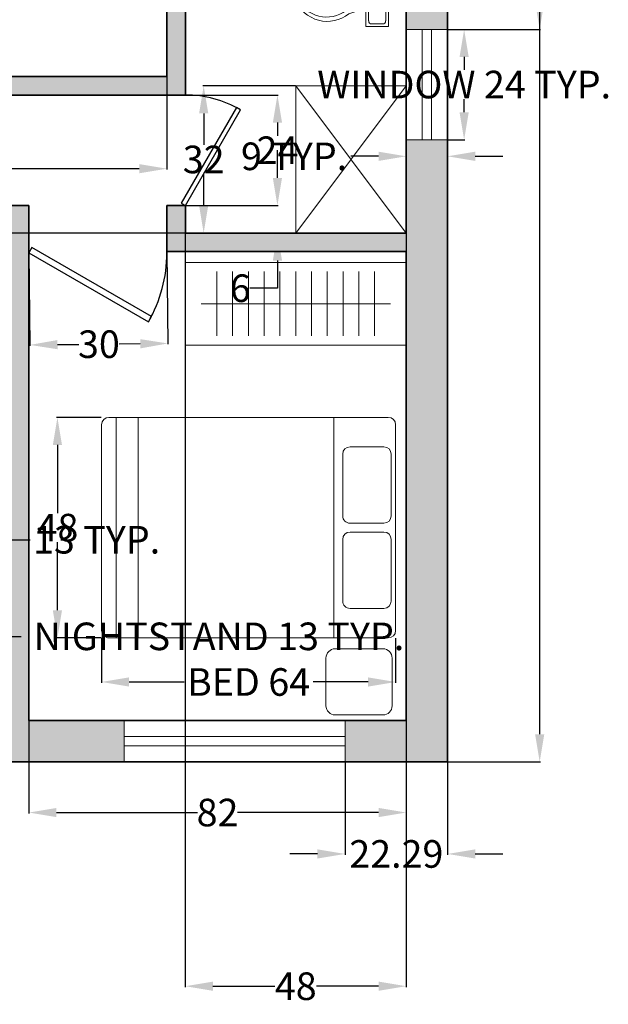
# Model space of a CAD drawing. Units: inches. Extents: x -26 to 363, y -399 to 37.
# Tile 2 of 4: x 232 to 360, y -399 to -185. Entities that reach past the tile are written whole.
import ezdxf

# ---------------------------------------------------------------- set-up
doc = ezdxf.new("R2010")
doc.units = ezdxf.units.IN
doc.header["$MEASUREMENT"] = 0
for name, color, linetype, lineweight in [('A-ANNO-DIMS', 2, 'Continuous', 18), ('A-DOOR', 3, 'Continuous', 25), ('A-FLOR-CASE', 8, 'Continuous', 18), ('A-FLOR-FIXT', 9, 'Continuous', 18), ('A-FURN', 8, 'Continuous', 18), ('A-GLAZ', 4, 'Continuous', 18), ('A-WALL', 7, 'Continuous', 35), ('A-WALL-PATT', 251, 'Continuous', 13)]:
    doc.layers.add(name, color=color, linetype=linetype, lineweight=lineweight)
doc.styles.get("Standard").update_dxf_attribs({"font": 'arial.ttf'})
doc.dimstyles.get("Standard").update_dxf_attribs({"dimtxt": 6, "dimasz": 6, "dimexe": 0.18, "dimexo": 0.0625, "dimgap": 0.09, "dimtad": 0, "dimtih": 1, "dimtoh": 1, "dimdec": 0, "dimzin": 0, "dimdsep": 46, "dimlunit": 4, "dimtxsty": 'Standard', "dimcen": 0.09, "dimadec": 0, "dimazin": 0, "dimtfac": 1, "dimtdec": 0, "dimtofl": 0, "dimtmove": 0, "dimatfit": 3, "dimfxl": 1, "dimtolj": 1, "dimtzin": 0, "dimarcsym": 0})

# ---------------------------------------------------------------- blocks, each defined once
blk = doc.blocks.new('*U3')
for p, q in [((0, 0), (0, 6)), ((40, 0), (40, 6))]:
    blk.add_line(p, q)
blk.add_lwpolyline([(0, 0), (34.64, -20), (35.52, -18.48), (0.87, 1.52)], close=True)
blk.add_arc((0, 0), 40, 330, 0)
blk = doc.blocks.new('Toilet - top')
for p, q in [((9.5, -6), (9.5, -2)), ((-10, -8.5), (-8, -8.5)), ((-10, -9.5), (-10, -8.5)), ((-7, -9.5), (-10, -9.5)), ((-8, -8.5), (-8, -8)), ((-7, -8), (-7, -9.5)), ((-4, -8), (-6, -14)), ((4, -8), (6, -14)), ((4, -14), (-4, -14))]:
    blk.add_line(p, q)
blk.add_lwpolyline([(10.5, -8), (10.5, 0), (-10.5, 0), (-10.5, -8)], close=True)
for points in [[(-9.5, -2), (-9.5, -6)], [(8.5, -1), (-8.5, -1)], [(-8.5, -7), (8.5, -7)]]:
    blk.add_lwpolyline(points)
for centre, radius, start, end in [((-8.62, -1.88), 0.884, 81.8699, 188.1301), ((8.62, -1.88), 0.884, 351.8699, 98.1301), ((-8.62, -6.12), 0.884, 171.8699, 278.1301), ((8.62, -6.12), 0.884, 261.8699, 8.1301), ((3.52, -21.58), 12.17, 141.4691, 247.9714), ((4.2, -21.82), 11.33, 136.3677, 238.9468), ((-3.52, -21.58), 12.17, 292.0284, 38.5307), ((-4.2, -21.82), 11.33, 301.053, 43.6321), ((0, -27.88), 4, 245.7318, 294.2682), ((0, -29), 4, 254.8605, 285.1395)]:
    blk.add_arc(centre, radius, start, end)
blk = doc.blocks.new('Bed - Queen')
for p, q in [((2, 0), (57.99999, 0)), ((0, -78.00003), (0, -2)), ((9.99999, -1.2), (26.79998, -1.2)), ((33.19999, -1.2), (49.99999, -1.2)), ((59.99999, -2), (59.99999, -78.00003)), ((7.99999, -12.4), (7.99999, -3.2)), ((28.79998, -3.2), (28.79998, -12.4)), ((31.19999, -12.4), (31.19999, -3.2)), ((51.99999, -3.2), (51.99999, -12.4)), ((9.99999, -14.4), (26.79998, -14.4)), ((33.19999, -14.4), (49.99999, -14.4)), ((59.99999, -16.8), (0, -16.8)), ((59.99999, -70.00003), (0, -70.00003)), ((59.99999, -76.00003), (0, -76.00003)), ((57.99999, -80.00003), (2, -80.00003))]:
    blk.add_line(p, q)
for centre, start, end in [((2, -2), 90, 180), ((57.99999, -2), 0, 90), ((9.99999, -3.2), 90, 180), ((26.79998, -3.2), 0, 90), ((33.19999, -3.2), 90, 180), ((49.99999, -3.2), 0, 90), ((9.99999, -12.4), 180, 270), ((26.79998, -12.4), 270, 0), ((33.19999, -12.4), 180, 270), ((49.99999, -12.4), 270, 0), ((2, -78.00003), 180, 270), ((57.99999, -78.00003), 270, 0)]:
    blk.add_arc(centre, 2, start, end)
blk = doc.blocks.new('WIN-48IN')
for p, q in [((0, 0), (0, 9)), ((48, 9), (48, 0)), ((48, 5.5), (0, 5.5)), ((48, 3.5), (0, 3.5))]:
    blk.add_line(p, q)
blk = doc.blocks.new('WIN-24IN')
for p, q in [((0, 24), (9, 24)), ((3.5, 24), (3.5, 0)), ((5.5, 24), (5.5, 0)), ((9, 0), (0, 0))]:
    blk.add_line(p, q)
blk = doc.blocks.new('*D23')
at = {"layer": 'A-ANNO-DIMS', "color": 0, "lineweight": -2, "transparency": 16777216}
for p, q in [((250.11, -319.65), (250.11, -329.36)), ((314.03, -319.65), (314.03, -329.36)), ((256.11, -329.18), (268.05, -329.18)), ((308.03, -329.18), (296.09, -329.18))]:
    blk.add_line(p, q, dxfattribs=at)
at = {"layer": 'A-ANNO-DIMS', "color": 0, "transparency": 16777216}
for points in [[(256.11, -328.18), (256.11, -330.18), (250.11, -329.18)], [(308.03, -328.18), (308.03, -330.18), (314.03, -329.18)]]:
    blk.add_solid(points, dxfattribs=at)
at = {"layer": 'Defpoints', "color": 0, "transparency": 16777216}
for p in [(250.11, -319.59), (314.03, -319.59), (314.03, -329.18)]:
    blk.add_point(p, dxfattribs=at)
at = {"layer": 'A-ANNO-DIMS', "color": 0, "transparency": 16777216, "insert": (282.07, -329.18), "char_height": 6, "attachment_point": 5}
blk.add_mtext('\\A1;BED 64', dxfattribs=at)
blk = doc.blocks.new('*D24')
at = {"layer": 'A-ANNO-DIMS', "color": 0, "lineweight": -2, "transparency": 16777216}
for p, q in [((250.04, -271.64), (240.34, -271.64)), ((240.52, -277.64), (240.52, -292.46)), ((240.52, -313.59), (240.52, -298.77)), ((250.04, -319.59), (240.34, -319.59))]:
    blk.add_line(p, q, dxfattribs=at)
at = {"layer": 'A-ANNO-DIMS', "color": 0, "transparency": 16777216}
for points in [[(239.52, -277.64), (241.52, -277.64), (240.52, -271.64)], [(239.52, -313.59), (241.52, -313.59), (240.52, -319.59)]]:
    blk.add_solid(points, dxfattribs=at)
at = {"layer": 'Defpoints', "color": 0, "transparency": 16777216}
for p in [(250.11, -271.64), (240.52, -319.59), (250.11, -319.59)]:
    blk.add_point(p, dxfattribs=at)
at = {"layer": 'A-ANNO-DIMS', "color": 0, "transparency": 16777216, "insert": (240.52, -295.62), "char_height": 6, "attachment_point": 5}
blk.add_mtext('\\A1;48', dxfattribs=at)
blk = doc.blocks.new('*D29')
at = {"layer": 'A-ANNO-DIMS', "color": 0, "lineweight": -2, "transparency": 16777216}
for p, q in [((325.39, -187.28), (329.1, -187.28)), ((328.92, -193.28), (328.92, -196.09)), ((328.92, -205.28), (328.92, -202.48)), ((325.39, -211.28), (329.1, -211.28))]:
    blk.add_line(p, q, dxfattribs=at)
at = {"layer": 'A-ANNO-DIMS', "color": 0, "transparency": 16777216}
for points in [[(327.92, -193.28), (329.92, -193.28), (328.92, -187.28)], [(327.92, -205.28), (329.92, -205.28), (328.92, -211.28)]]:
    blk.add_solid(points, dxfattribs=at)
at = {"layer": 'Defpoints', "color": 0, "transparency": 16777216}
for p in [(325.32, -187.28), (325.32, -211.28), (328.92, -211.28)]:
    blk.add_point(p, dxfattribs=at)
at = {"layer": 'A-ANNO-DIMS', "color": 0, "transparency": 16777216, "insert": (328.92, -199.28), "char_height": 6, "attachment_point": 5}
blk.add_mtext('\\A1;WINDOW 24 TYP.', dxfattribs=at)
blk = doc.blocks.new('*D30')
at = {"layer": 'A-ANNO-DIMS', "color": 0, "lineweight": -2, "transparency": 16777216}
for p, q in [((316.32, -211.35), (316.32, -215.06)), ((325.32, -211.35), (325.32, -215.06)), ((310.32, -214.88), (304.32, -214.88)), ((331.32, -214.88), (337.32, -214.88))]:
    blk.add_line(p, q, dxfattribs=at)
at = {"layer": 'A-ANNO-DIMS', "color": 0, "transparency": 16777216}
for points in [[(310.32, -213.88), (310.32, -215.88), (316.32, -214.88)], [(331.32, -213.88), (331.32, -215.88), (325.32, -214.88)]]:
    blk.add_solid(points, dxfattribs=at)
at = {"layer": 'Defpoints', "color": 0, "transparency": 16777216}
for p in [(316.32, -211.28), (325.32, -211.28), (316.32, -214.88)]:
    blk.add_point(p, dxfattribs=at)
at = {"layer": 'A-ANNO-DIMS', "color": 0, "transparency": 16777216, "insert": (291.96, -214.88), "char_height": 6, "attachment_point": 5}
blk.add_mtext('\\A1;9 TYP.', dxfattribs=at)
blk = doc.blocks.new('*D31')
at = {"layer": 'A-ANNO-DIMS', "color": 0, "lineweight": -2, "transparency": 16777216}
for p, q in [((213.62, -317.36), (213.62, -319.44)), ((226.67, -317.36), (226.67, -319.44)), ((219.62, -319.26), (220.67, -319.26)), ((226.67, -319.26), (232.67, -319.26))]:
    blk.add_line(p, q, dxfattribs=at)
at = {"layer": 'A-ANNO-DIMS', "color": 0, "transparency": 16777216}
for points in [[(219.62, -318.26), (219.62, -320.26), (213.62, -319.26)], [(220.67, -318.26), (220.67, -320.26), (226.67, -319.26)]]:
    blk.add_solid(points, dxfattribs=at)
at = {"layer": 'Defpoints', "color": 0, "transparency": 16777216}
for p in [(213.62, -317.3), (226.67, -317.3), (226.67, -319.26)]:
    blk.add_point(p, dxfattribs=at)
at = {"layer": 'A-ANNO-DIMS', "color": 0, "transparency": 16777216, "insert": (275.62, -319.26), "char_height": 6, "attachment_point": 5}
blk.add_mtext('\\A1;NIGHTSTAND 13 TYP.', dxfattribs=at)
blk = doc.blocks.new('*D32')
at = {"layer": 'A-ANNO-DIMS', "color": 0, "lineweight": -2, "transparency": 16777216}
for p, q in [((228.63, -304.25), (228.63, -298.25)), ((228.63, -298.25), (234.63, -298.25)), ((226.73, -304.25), (228.81, -304.25)), ((228.63, -311.3), (228.63, -310.25)), ((226.73, -317.3), (228.81, -317.3))]:
    blk.add_line(p, q, dxfattribs=at)
at = {"layer": 'A-ANNO-DIMS', "color": 0, "transparency": 16777216}
for points in [[(227.63, -310.25), (229.63, -310.25), (228.63, -304.25)], [(227.63, -311.3), (229.63, -311.3), (228.63, -317.3)]]:
    blk.add_solid(points, dxfattribs=at)
at = {"layer": 'Defpoints', "color": 0, "transparency": 16777216}
for p in [(226.67, -304.25), (228.63, -304.25), (226.67, -317.3)]:
    blk.add_point(p, dxfattribs=at)
at = {"layer": 'A-ANNO-DIMS', "color": 0, "transparency": 16777216, "insert": (249.04, -298.25), "char_height": 6, "attachment_point": 5}
blk.add_mtext('\\A1;13 TYP.', dxfattribs=at)
blk = doc.blocks.new('*D41')
at = {"layer": 'A-ANNO-DIMS', "color": 0, "lineweight": -2, "transparency": 16777216}
for p, q in [((325.39, 13.44), (345.52, 13.44)), ((345.34, 7.44), (345.34, -163.4)), ((345.34, -340.56), (345.34, -169.71)), ((325.39, -346.56), (345.52, -346.56))]:
    blk.add_line(p, q, dxfattribs=at)
at = {"layer": 'A-ANNO-DIMS', "color": 0, "transparency": 16777216}
for points in [[(344.34, 7.44), (346.34, 7.44), (345.34, 13.44)], [(344.34, -340.56), (346.34, -340.56), (345.34, -346.56)]]:
    blk.add_solid(points, dxfattribs=at)
at = {"layer": 'Defpoints', "color": 0, "transparency": 16777216}
for p in [(325.32, 13.44), (345.34, 13.44), (325.32, -346.56)]:
    blk.add_point(p, dxfattribs=at)
at = {"layer": 'A-ANNO-DIMS', "color": 0, "transparency": 16777216, "insert": (345.34, -166.56), "char_height": 6, "attachment_point": 5}
blk.add_mtext('\\A1;360', dxfattribs=at)
blk = doc.blocks.new('*D47')
at = {"layer": 'A-ANNO-DIMS', "color": 0, "lineweight": -2, "transparency": 16777216}
for p, q in [((176.32, -197.62), (176.32, -217.75)), ((264.32, -197.62), (264.32, -217.75)), ((182.32, -217.57), (215.93, -217.57)), ((258.32, -217.57), (224.72, -217.57))]:
    blk.add_line(p, q, dxfattribs=at)
at = {"layer": 'A-ANNO-DIMS', "color": 0, "transparency": 16777216}
for points in [[(182.32, -216.57), (182.32, -218.57), (176.32, -217.57)], [(258.32, -216.57), (258.32, -218.57), (264.32, -217.57)]]:
    blk.add_solid(points, dxfattribs=at)
at = {"layer": 'Defpoints', "color": 0, "transparency": 16777216}
for p in [(176.32, -197.56), (264.32, -197.56), (176.32, -217.57)]:
    blk.add_point(p, dxfattribs=at)
at = {"layer": 'A-ANNO-DIMS', "color": 0, "transparency": 16777216, "insert": (220.32, -217.57), "char_height": 6, "attachment_point": 5}
blk.add_mtext('\\A1;88', dxfattribs=at)
blk = doc.blocks.new('*D49')
at = {"layer": 'A-ANNO-DIMS', "color": 0, "lineweight": -2, "transparency": 16777216}
for p, q in [((268.32, -231.62), (268.32, -395.51)), ((316.32, -231.62), (316.32, -395.51)), ((274.32, -395.33), (287.81, -395.33)), ((310.32, -395.33), (296.84, -395.33))]:
    blk.add_line(p, q, dxfattribs=at)
at = {"layer": 'A-ANNO-DIMS', "color": 0, "transparency": 16777216}
for points in [[(274.32, -394.33), (274.32, -396.33), (268.32, -395.33)], [(310.32, -394.33), (310.32, -396.33), (316.32, -395.33)]]:
    blk.add_solid(points, dxfattribs=at)
at = {"layer": 'Defpoints', "color": 0, "transparency": 16777216}
for p in [(268.32, -231.56), (316.32, -231.56), (316.32, -395.33)]:
    blk.add_point(p, dxfattribs=at)
at = {"layer": 'A-ANNO-DIMS', "color": 0, "transparency": 16777216, "insert": (292.32, -395.33), "char_height": 6, "attachment_point": 5}
blk.add_mtext('\\A1;48', dxfattribs=at)
blk = doc.blocks.new('*D51')
at = {"layer": 'A-ANNO-DIMS', "color": 0, "lineweight": -2, "transparency": 16777216}
for p, q in [((268.26, -167.56), (5.13, -167.56)), ((5.31, -173.56), (5.31, -196.4)), ((5.31, -225.56), (5.31, -202.71)), ((268.26, -231.56), (5.13, -231.56))]:
    blk.add_line(p, q, dxfattribs=at)
at = {"layer": 'A-ANNO-DIMS', "color": 0, "transparency": 16777216}
for points in [[(4.31, -173.56), (6.31, -173.56), (5.31, -167.56)], [(4.31, -225.56), (6.31, -225.56), (5.31, -231.56)]]:
    blk.add_solid(points, dxfattribs=at)
at = {"layer": 'Defpoints', "color": 0, "transparency": 16777216}
for p in [(268.32, -167.56), (5.31, -231.56), (268.32, -231.56)]:
    blk.add_point(p, dxfattribs=at)
at = {"layer": 'A-ANNO-DIMS', "color": 0, "transparency": 16777216, "insert": (5.31, -199.56), "char_height": 6, "attachment_point": 5}
blk.add_mtext('\\A1;64', dxfattribs=at)
blk = doc.blocks.new('*D52')
at = {"layer": 'A-ANNO-DIMS', "color": 0, "lineweight": -2, "transparency": 16777216}
for p, q in [((234.32, -337.62), (234.32, -357.75)), ((316.32, -337.62), (316.32, -357.75)), ((240.32, -357.57), (270.96, -357.57)), ((310.32, -357.57), (279.68, -357.57))]:
    blk.add_line(p, q, dxfattribs=at)
at = {"layer": 'A-ANNO-DIMS', "color": 0, "transparency": 16777216}
for points in [[(240.32, -356.57), (240.32, -358.57), (234.32, -357.57)], [(310.32, -356.57), (310.32, -358.57), (316.32, -357.57)]]:
    blk.add_solid(points, dxfattribs=at)
at = {"layer": 'Defpoints', "color": 0, "transparency": 16777216}
for p in [(234.32, -337.56), (316.32, -337.56), (234.32, -357.57)]:
    blk.add_point(p, dxfattribs=at)
at = {"layer": 'A-ANNO-DIMS', "color": 0, "transparency": 16777216, "insert": (275.32, -357.57), "char_height": 6, "attachment_point": 5}
blk.add_mtext('\\A1;82', dxfattribs=at)
blk = doc.blocks.new('*D56')
at = {"layer": 'A-ANNO-DIMS', "color": 0, "lineweight": -2, "transparency": 16777216}
for p, q in [((303.03, -346.62), (303.03, -366.75)), ((325.32, -346.62), (325.32, -366.75)), ((297.03, -366.57), (291.03, -366.57)), ((331.32, -366.57), (337.32, -366.57))]:
    blk.add_line(p, q, dxfattribs=at)
at = {"layer": 'A-ANNO-DIMS', "color": 0, "transparency": 16777216}
for points in [[(297.03, -365.57), (297.03, -367.57), (303.03, -366.57)], [(331.32, -365.57), (331.32, -367.57), (325.32, -366.57)]]:
    blk.add_solid(points, dxfattribs=at)
at = {"layer": 'Defpoints', "color": 0, "transparency": 16777216}
for p in [(303.03, -346.56), (325.32, -346.56), (303.03, -366.57)]:
    blk.add_point(p, dxfattribs=at)
at = {"layer": 'A-ANNO-DIMS', "color": 0, "transparency": 16777216, "insert": (314.18, -366.57), "char_height": 6, "attachment_point": 5}
blk.add_mtext('\\A1;22.29', dxfattribs=at)
blk = doc.blocks.new('*D58')
at = {"layer": 'A-ANNO-DIMS', "color": 0, "lineweight": -2, "transparency": 16777216}
for p, q in [((316.39, -167.56), (345.52, -167.56)), ((345.34, -173.56), (345.34, -174.26)), ((345.34, -181.28), (345.34, -180.58)), ((325.39, -187.28), (345.52, -187.28))]:
    blk.add_line(p, q, dxfattribs=at)
at = {"layer": 'A-ANNO-DIMS', "color": 0, "transparency": 16777216}
for points in [[(344.34, -173.56), (346.34, -173.56), (345.34, -167.56)], [(344.34, -181.28), (346.34, -181.28), (345.34, -187.28)]]:
    blk.add_solid(points, dxfattribs=at)
at = {"layer": 'Defpoints', "color": 0, "transparency": 16777216}
for p in [(316.32, -167.56), (345.34, -167.56), (325.32, -187.28)]:
    blk.add_point(p, dxfattribs=at)
at = {"layer": 'A-ANNO-DIMS', "color": 0, "transparency": 16777216, "insert": (345.34, -177.42), "char_height": 6, "attachment_point": 5}
blk.add_mtext('\\A1;19.73', dxfattribs=at)
blk = doc.blocks.new('*D64')
at = {"layer": 'A-ANNO-DIMS', "color": 0, "lineweight": -2, "transparency": 16777216}
for p, q in [((268.39, -201.56), (288.52, -201.56)), ((288.34, -207.56), (288.34, -210.45)), ((288.34, -219.56), (288.34, -216.66)), ((268.39, -225.56), (288.52, -225.56))]:
    blk.add_line(p, q, dxfattribs=at)
at = {"layer": 'A-ANNO-DIMS', "color": 0, "transparency": 16777216}
for points in [[(287.34, -207.56), (289.34, -207.56), (288.34, -201.56)], [(287.34, -219.56), (289.34, -219.56), (288.34, -225.56)]]:
    blk.add_solid(points, dxfattribs=at)
at = {"layer": 'Defpoints', "color": 0, "transparency": 16777216}
for p in [(268.32, -201.56), (268.32, -225.56), (288.34, -225.56)]:
    blk.add_point(p, dxfattribs=at)
at = {"layer": 'A-ANNO-DIMS', "color": 0, "transparency": 16777216, "insert": (288.34, -213.56), "char_height": 6, "attachment_point": 5}
blk.add_mtext('\\A1;24', dxfattribs=at)
blk = doc.blocks.new('*D65')
at = {"layer": 'A-ANNO-DIMS', "color": 0, "lineweight": -2, "transparency": 16777216}
for p, q in [((234.32, -235.94), (234.54, -256.07)), ((264.32, -235.62), (264.54, -255.75)), ((240.54, -255.83), (245.16, -255.78)), ((258.54, -255.64), (253.91, -255.69))]:
    blk.add_line(p, q, dxfattribs=at)
at = {"layer": 'A-ANNO-DIMS', "color": 0, "transparency": 16777216}
for points in [[(258.53, -254.64), (258.55, -256.64), (264.54, -255.57)], [(240.53, -254.83), (240.55, -256.83), (234.54, -255.89)]]:
    blk.add_solid(points, dxfattribs=at)
at = {"layer": 'Defpoints', "color": 0, "transparency": 16777216}
for p in [(234.32, -235.88), (264.32, -235.56), (234.54, -255.89)]:
    blk.add_point(p, dxfattribs=at)
at = {"layer": 'A-ANNO-DIMS', "color": 0, "transparency": 16777216, "insert": (249.54, -255.73), "char_height": 6, "attachment_point": 5}
blk.add_mtext('\\A1;30', dxfattribs=at)
blk = doc.blocks.new('*D68')
at = {"layer": 'A-ANNO-DIMS', "color": 0, "lineweight": -2, "transparency": 16777216}
for p, q in [((292.26, -199.56), (272.13, -199.56)), ((272.31, -205.56), (272.31, -212.4)), ((272.31, -225.56), (272.31, -218.71)), ((292.26, -231.56), (272.13, -231.56))]:
    blk.add_line(p, q, dxfattribs=at)
at = {"layer": 'A-ANNO-DIMS', "color": 0, "transparency": 16777216}
for points in [[(271.31, -205.56), (273.31, -205.56), (272.31, -199.56)], [(271.31, -225.56), (273.31, -225.56), (272.31, -231.56)]]:
    blk.add_solid(points, dxfattribs=at)
at = {"layer": 'Defpoints', "color": 0, "transparency": 16777216}
for p in [(272.31, -199.56), (292.32, -199.56), (292.32, -231.56)]:
    blk.add_point(p, dxfattribs=at)
at = {"layer": 'A-ANNO-DIMS', "color": 0, "transparency": 16777216, "insert": (272.31, -215.56), "char_height": 6, "attachment_point": 5}
blk.add_mtext('\\A1;32', dxfattribs=at)
blk = doc.blocks.new('*D78')
at = {"layer": 'A-ANNO-DIMS', "color": 0, "lineweight": -2, "transparency": 16777216}
for p, q in [((288.34, -219.56), (288.34, -213.56)), ((268.39, -225.56), (288.52, -225.56)), ((268.39, -231.56), (288.52, -231.56)), ((288.34, -237.56), (288.34, -243.56)), ((288.34, -243.56), (282.34, -243.56))]:
    blk.add_line(p, q, dxfattribs=at)
at = {"layer": 'A-ANNO-DIMS', "color": 0, "transparency": 16777216}
for points in [[(287.34, -219.56), (289.34, -219.56), (288.34, -225.56)], [(287.34, -237.56), (289.34, -237.56), (288.34, -231.56)]]:
    blk.add_solid(points, dxfattribs=at)
at = {"layer": 'Defpoints', "color": 0, "transparency": 16777216}
for p in [(268.32, -225.56), (268.32, -231.56), (288.34, -231.56)]:
    blk.add_point(p, dxfattribs=at)
at = {"layer": 'A-ANNO-DIMS', "color": 0, "transparency": 16777216, "insert": (280.27, -243.56), "char_height": 6, "attachment_point": 5}
blk.add_mtext('\\A1;6', dxfattribs=at)

msp = doc.modelspace()

# ---------------------------------------------------------------- hatches: boundary and pattern name
at = {"layer": 'A-WALL-PATT'}
h = msp.add_hatch(color=256, dxfattribs=at)
h.dxf.hatch_style = 1
h.paths.add_polyline_path([(325.3228, -139.9712), (316.3228, -139.9712), (316.3228, -163.5551), (292.3228, -163.5551), (268.3228, -163.5551), (268.3228, -91.5551), (274.3228, -91.5551), (274.3228, -87.5551), (172.3228, -87.5551), (172.3228, -91.5551), (172.3228, -97.5551), (176.3228, -97.5551), (176.3228, -91.5551), (264.3228, -91.5551), (264.3228, -197.5551), (258.3228, -197.5551), (176.3228, -197.5551), (176.3228, -127.5551), (172.3228, -127.5551), (172.3228, -197.5551), (172.3228, -201.5551), (258.3228, -201.5551), (264.3228, -201.5551), (268.3228, -201.5551), (268.3228, -167.5551), (316.3228, -167.5551), (316.3228, -187.2842), (325.3228, -187.2842)])
h = msp.add_hatch(color=256, dxfattribs=at)
h.dxf.hatch_style = 1
h.paths.add_polyline_path([(255.0334, -337.5551), (234.3228, -337.5551), (234.3228, -225.5551), (230.3228, -225.5551), (230.3228, -337.5551), (213.7273, -337.5551), (213.7273, -346.5551), (216.3228, -346.5551), (216.3228, -371.3126), (80.3228, -371.3126), (80.3228, -315.3126), (132.3228, -315.3126), (132.3228, -337.5551), (132.3228, -346.5551), (165.7273, -346.5551), (165.7273, -337.5551), (136.3228, -337.5551), (136.3228, -201.5551), (142.3228, -201.5551), (142.3228, -197.5551), (132.3228, -197.5551), (132.3228, -306.3126), (76.3228, -306.3126), (76.3228, -315.3126), (76.3228, -375.3126), (220.3228, -375.3126), (220.3228, -346.5551), (255.0334, -346.5551)])
h = msp.add_hatch(color=256, dxfattribs=at)
h.dxf.hatch_style = 1
h.paths.add_polyline_path([(325.3228, -211.2842), (316.3228, -211.2842), (316.3228, -231.5551), (292.3228, -231.5551), (268.3228, -231.5551), (268.3228, -225.5551), (264.3228, -225.5551), (264.3228, -235.5551), (316.3228, -235.5551), (316.3228, -337.5551), (303.0334, -337.5551), (303.0334, -346.5551), (325.3228, -346.5551)])

# ---------------------------------------------------------------- linework, layer by layer
at = {"layer": 'A-FLOR-CASE'}
for p, q in [((268.3228, -255.9392), (268.3228, -237.9392)), ((268.3228, -237.9392), (316.3228, -237.9392)), ((268.3228, -237.9392), (268.3228, -255.9392)), ((316.3228, -237.9392), (316.3228, -255.9392)), ((275.1799, -239.9392), (275.1799, -253.9392)), ((278.6085, -239.9392), (278.6085, -253.9392)), ((282.0371, -239.9392), (282.0371, -253.9392)), ((285.4656, -239.9392), (285.4656, -253.9392)), ((288.8942, -239.9392), (288.8942, -253.9392)), ((292.3228, -239.9392), (292.3228, -253.9392)), ((295.7513, -239.9392), (295.7513, -253.9392)), ((299.1799, -239.9392), (299.1799, -253.9392)), ((302.6085, -239.9392), (302.6085, -253.9392)), ((306.0371, -239.9392), (306.0371, -253.9392)), ((309.4656, -239.9392), (309.4656, -253.9392)), ((312.8942, -246.9392), (271.7513, -246.9392)), ((316.3228, -255.9392), (268.3228, -255.9392))]:
    msp.add_line(p, q, dxfattribs=at)
at = {"layer": 'A-FLOR-FIXT'}
for p, q in [((292.3228, -199.5551), (316.3228, -231.5551)), ((316.3228, -199.5551), (292.3228, -231.5551))]:
    msp.add_line(p, q, dxfattribs=at)
msp.add_lwpolyline([(316.3228, -199.5551), (292.3228, -199.5551), (292.3228, -231.5551), (316.3228, -231.5551)], close=True, dxfattribs=at)
at = {"layer": 'A-FURN'}
msp.add_lwpolyline([(311.2752, -336.3489), (300.8917, -336.3489, -0.41421356), (298.8917, -334.3489), (298.8917, -323.9654, -0.41421356), (300.8917, -321.9654), (311.2752, -321.9654, -0.41421356), (313.2752, -323.9654), (313.2752, -334.3489, -0.41421356)], format="xyb", close=True, dxfattribs=at)
at = {"layer": 'A-WALL'}
for p, q in [((264.3228, -91.5551), (264.3228, -197.5551)), ((268.3228, -167.5551), (268.3228, -201.5551)), ((316.3228, -167.5551), (316.3228, -231.5551)), ((258.3228, -197.5551), (176.3228, -197.5551)), ((264.3228, -197.5551), (258.3228, -197.5551)), ((258.3228, -201.5551), (172.3228, -201.5551)), ((264.3228, -201.5551), (258.3228, -201.5551)), ((268.3228, -201.5551), (264.3228, -201.5551)), ((234.3228, -225.5551), (230.3228, -225.5551)), ((234.3228, -225.5551), (234.3228, -337.5551)), ((264.3228, -225.5551), (264.3228, -235.5551)), ((268.3228, -225.5551), (264.3228, -225.5551)), ((268.3228, -225.5551), (268.3228, -231.5551)), ((268.3228, -231.5551), (316.3228, -231.5551)), ((264.3228, -235.5551), (316.3228, -235.5551)), ((316.3228, -235.5551), (316.3228, -337.5551)), ((316.3228, -337.5551), (234.3228, -337.5551))]:
    msp.add_line(p, q, dxfattribs=at)
msp.add_lwpolyline([(25.3228, -315.3126), (25.3228, 13.4449), (325.3228, 13.4449), (325.3228, -346.5551), (220.3228, -346.5551)], dxfattribs=at)

# ---------------------------------------------------------------- block references
at = {"layer": 'A-DOOR', "xscale": 0.6, "yscale": 0.6, "zscale": 0.6, "rotation": 90}
msp.add_blockref('*U3', (268.3228, -225.5551), dxfattribs=at)
at = {"layer": 'A-DOOR', "xscale": 0.75, "yscale": 0.75, "zscale": 0.75}
msp.add_blockref('*U3', (234.3228, -235.8792), dxfattribs=at)
at = {"layer": 'A-FLOR-FIXT', "xscale": 0.6163129826161287, "yscale": 0.6163129826161287, "zscale": 0.6163129826161287, "rotation": 270}
msp.add_blockref('Toilet - top', (312.4819, -180.2133), dxfattribs=at)
at = {"layer": 'A-FURN', "xscale": 0.7990837807536608, "yscale": 0.7990837807536608, "zscale": 0.7990837807536608, "rotation": 270}
msp.add_blockref('Bed - Queen', (314.0336, -271.6434), dxfattribs=at)
at = {"layer": 'A-GLAZ', "rotation": 180}
msp.add_blockref('WIN-24IN', (325.3225, -187.2844), dxfattribs=at)
at = {"layer": 'A-GLAZ'}
msp.add_blockref('WIN-48IN', (255.0334, -346.555), dxfattribs=at)

# ---------------------------------------------------------------- dimensions: what is measured, and where the dimension line sits
at = {"layer": 'A-ANNO-DIMS'}
for base, p1, p2, angle, override, picture, middle in [((345.3393, 13.4449), (325.3228, -346.5551), (325.3228, 13.4449), 90, {"dimdec": 0, "dimlfac": 1, "dimrnd": 0, "dimzin": 0, "dimdsep": 46, "dimlunit": 2}, '*D41', (345.3393, -166.5551)), ((5.3063, -231.5551), (268.3228, -167.5551), (268.3228, -231.5551), 90, {"dimdec": 0, "dimlfac": 1, "dimrnd": 0, "dimzin": 0, "dimdsep": 46, "dimlunit": 2}, '*D51', (5.3063, -199.5551)), ((345.3393, -167.5551), (325.3228, -187.2842), (316.3228, -167.5551), 90, {"dimdec": 2, "dimlfac": 1, "dimrnd": 0, "dimzin": 0, "dimdsep": 46, "dimlunit": 2}, '*D58', (345.3393, -177.4197)), ((176.3228, -217.5716), (264.3228, -197.5551), (176.3228, -197.5551), 180, {"dimdec": 0, "dimlfac": 1, "dimrnd": 0, "dimzin": 0, "dimdsep": 46, "dimlunit": 2}, '*D47', (220.3228, -217.5716)), ((272.3063, -199.5551), (292.3228, -231.5551), (292.3228, -199.5551), 90, {"dimdec": 0, "dimlfac": 1, "dimrnd": 0, "dimzin": 0, "dimdsep": 46, "dimlunit": 2}, '*D68', (272.3063, -215.5551)), ((288.3393, -225.5551), (268.3228, -201.5551), (268.3228, -225.5551), 270, {"dimdec": 0, "dimlfac": 1, "dimrnd": 0, "dimzin": 0, "dimdsep": 46, "dimlunit": 2}, '*D64', (288.3393, -213.5551)), ((288.3393, -231.5551), (268.3228, -225.5551), (268.3228, -231.5551), 270, {"dimdec": 0, "dimlfac": 1, "dimrnd": 0, "dimzin": 0, "dimdsep": 46, "dimlunit": 2}, '*D78', (280.2684, -243.5551)), ((234.539, -255.8945), (264.3228, -235.5551), (234.3228, -235.8792), 180.618876, {"dimdec": 0, "dimlfac": 1, "dimrnd": 0, "dimzin": 0, "dimdsep": 46, "dimlunit": 2}, '*D65', (249.539, -255.7325)), ((240.5179, -319.5884), (250.1069, -271.6434), (250.1069, -319.5884), 270, {"dimdec": 0, "dimlfac": 1, "dimrnd": 0, "dimzin": 0, "dimdsep": 46, "dimlunit": 2}, '*D24', (240.5179, -295.6159)), ((234.3228, -357.5716), (316.3228, -337.5551), (234.3228, -337.5551), 180, {"dimdec": 0, "dimlfac": 1, "dimrnd": 0, "dimzin": 0, "dimdsep": 46, "dimlunit": 2}, '*D52', (275.3228, -357.5716)), ((303.0334, -366.5716), (325.3228, -346.5551), (303.0334, -346.5551), 180, {"dimdec": 2, "dimlfac": 1, "dimrnd": 0, "dimzin": 0, "dimdsep": 46, "dimlunit": 2}, '*D56', (314.1781, -366.5716))]:
    dim = msp.add_linear_dim(base=base, p1=p1, p2=p2, angle=angle, dimstyle='Standard', override=override, dxfattribs=at)
    dim.commit()
    dim.dimension.update_dxf_attribs({"geometry": picture, "text_midpoint": middle})
for base, p1, p2, angle, text, picture, middle in [((328.9228, -211.2842), (325.3228, -187.2842), (325.3228, -211.2842), 270, 'WINDOW <> TYP.', '*D29', (328.9228, -199.2842)), ((316.3228, -214.8842), (325.3228, -211.2842), (316.3228, -211.2842), 180, '<> TYP.', '*D30', (291.9606, -214.8842)), ((228.629, -304.2468), (226.6713, -317.298), (226.6713, -304.2468), 90, '<> TYP.', '*D32', (249.0396, -298.2468))]:
    dim = msp.add_linear_dim(base=base, p1=p1, p2=p2, angle=angle, text=text, dimstyle='Standard', override={"dimdec": 0, "dimlfac": 1, "dimrnd": 0, "dimzin": 0, "dimdsep": 46, "dimlunit": 2}, dxfattribs=at)
    dim.commit()
    dim.dimension.update_dxf_attribs({"geometry": picture, "text_midpoint": middle})
dim = msp.add_linear_dim(base=(316.3228, -395.3291), p1=(268.3228, -231.5551), p2=(316.3228, -231.5551), dimstyle='Standard', override={"dimdec": 0, "dimlfac": 1, "dimrnd": 0, "dimzin": 0, "dimdsep": 46, "dimlunit": 2}, dxfattribs=at)
dim.commit()
dim.dimension.update_dxf_attribs({"geometry": '*D49', "text_midpoint": (292.3228, -395.3291)})
for base, p1, p2, text, picture, middle in [((226.6713, -319.2556), (213.6202, -317.298), (226.6713, -317.298), 'NIGHTSTAND <> TYP.', '*D31', (275.6249, -319.2556)), ((314.0336, -329.1774), (250.1069, -319.5884), (314.0336, -319.5884), 'BED <>', '*D23', (282.0703, -329.1774))]:
    dim = msp.add_linear_dim(base=base, p1=p1, p2=p2, text=text, dimstyle='Standard', override={"dimdec": 0, "dimlfac": 1, "dimrnd": 0, "dimzin": 0, "dimdsep": 46, "dimlunit": 2}, dxfattribs=at)
    dim.commit()
    dim.dimension.update_dxf_attribs({"geometry": picture, "text_midpoint": middle})

doc.saveas('drawing.dxf')
